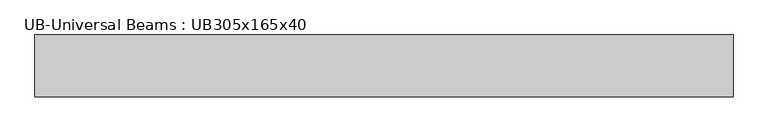
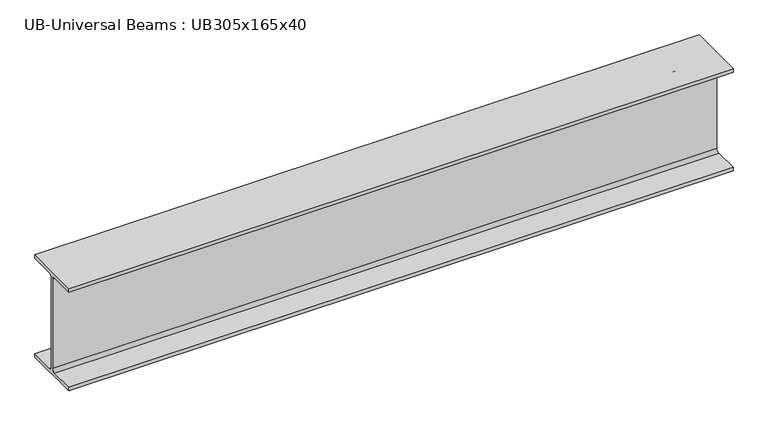
"""IFC4 building model written with IfcOpenShell, lengths in millimetres: beam geometry, UB-Universal Beams : UB305x165x40."""

from ifc_helpers import new_model, si_unit, point, frame, frame_2d, origin, place, context, project, spatial, polyline, circle_curve, trimmed, segment, composite_curve, outline, extrude, source, transform, mapped, element, save


def ub_universal_beams_ub305x165x40_5cbd381f(model_context):
    return source(origin(), model_context, "Body", "SweptSolid", [
        extrude(outline(composite_curve([segment(polyline([(82.5, -141.5), (82.5, -151.7), (-82.5, -151.7), (-82.5, -141.5), (-11.9, -141.5)]), True, "CONTINUOUS"), segment(trimmed(circle_curve(frame_2d((-11.9, -132.6)), 8.9), [point((-11.9, -141.5))], [point((-3.0, -132.6))], True, "CARTESIAN"), True, "CONTINUOUS"), segment(polyline([(-3.0, -132.6), (-3.0, 132.6)]), True, "CONTINUOUS"), segment(trimmed(circle_curve(frame_2d((-11.9, 132.6)), 8.9), [point((-3.0, 132.6))], [point((-11.9, 141.5))], True, "CARTESIAN"), True, "CONTINUOUS"), segment(polyline([(-11.9, 141.5), (-82.5, 141.5), (-82.5, 151.7), (82.5, 151.7), (82.5, 141.5), (11.9, 141.5)]), True, "CONTINUOUS"), segment(trimmed(circle_curve(frame_2d((11.9, 132.6)), 8.9), [point((11.9, 141.5))], [point((3.0, 132.6))], True, "CARTESIAN"), True, "CONTINUOUS"), segment(polyline([(3.0, 132.6), (3.0, -132.6)]), True, "CONTINUOUS"), segment(trimmed(circle_curve(frame_2d((11.9, -132.6)), 8.9), [point((3.0, -132.6))], [point((11.9, -141.5))], True, "CARTESIAN"), True, "CONTINUOUS"), segment(polyline([(11.9, -141.5), (82.5, -141.5)]), True, "CONTINUOUS")], self_intersect=False)), frame((-1037.85, 0.0, 0.0), z_axis=(1.0, 0.0, 0.0), x_axis=(0.0, 1.0, 0.0)), (0.0, 0.0, 1.0), 1863.5),
    ])


if __name__ == "__main__":
    model = new_model("IFC4")
    model_context = context("Model", 3, world=origin())
    ifc_project = project(units=[si_unit("LENGTHUNIT", "METRE", prefix="MILLI")], contexts=[model_context])
    site = spatial("IfcSite", under=ifc_project)
    building = spatial("IfcBuilding", under=site)
    placement = place(None, origin())
    ub_universal_beams_ub305x165x40_shape = ub_universal_beams_ub305x165x40_5cbd381f(model_context)
    element("IfcBeam", 1, ObjectType="UB-Universal Beams : UB305x165x40", at=placement, inside=building, context=model_context, shape_type="MappedRepresentation", body=[
        mapped(ub_universal_beams_ub305x165x40_shape, transform((0.0, 0.0, 0.0), x_axis=(1.0, 0.0, 0.0), y_axis=(0.0, 1.0, 0.0), z_axis=(0.0, 0.0, 1.0))),
    ])
    save(model, "model.ifc")

# Revit data of these elements
# Type "UB-Universal Beams : UB305x165x40"
#   Section Name Key = "UB305X165X40"
#   Width = 16.5 cm
#   Web Thickness = 0.6 cm
#   Web Fillet = 0.89 cm
#   Warping Constant = 164000.0 cm⁶
#   Torsional Moment of Inertia = 14.70 cm⁴
#   Section Area = 51.3 cm²
#   Plastic Modulus weak axis = 142.0 cm³
#   Plastic Modulus strong axis = 623.0 cm³
#   Nominal Weight = 40.2999 kgf/m
#   Moment of Inertia weak axis = 764.00 cm⁴
#   Moment of Inertia strong axis = 8503.00 cm⁴
#   Height = 30.34 cm
#   Flange Thickness = 1.02 cm
#   Elastic Modulus weak axis = 92.6 cm³
#   Elastic Modulus strong axis = 560.0 cm³
#   Centroid Vertical = 15.17 cm
#   Centroid Horizontal = 8.25 cm
#   Bolt Spacing = 9.0 cm
#   Length [instance default] = 1500 mm
#   Structural Material [instance default] = Metal - Steel 43-275
#   Type Comments = ""
#   Assembly Code = ""
# Element 1 (IfcBeam, "UB-Universal Beams : UB305x165x40")
#   Materials on its faces: "Metal - Steel 43-275"
# Materials
#   "Metal - Steel 43-275": class "Metal", colour RGB 247 247 247, transparency 0, Cost = 0
